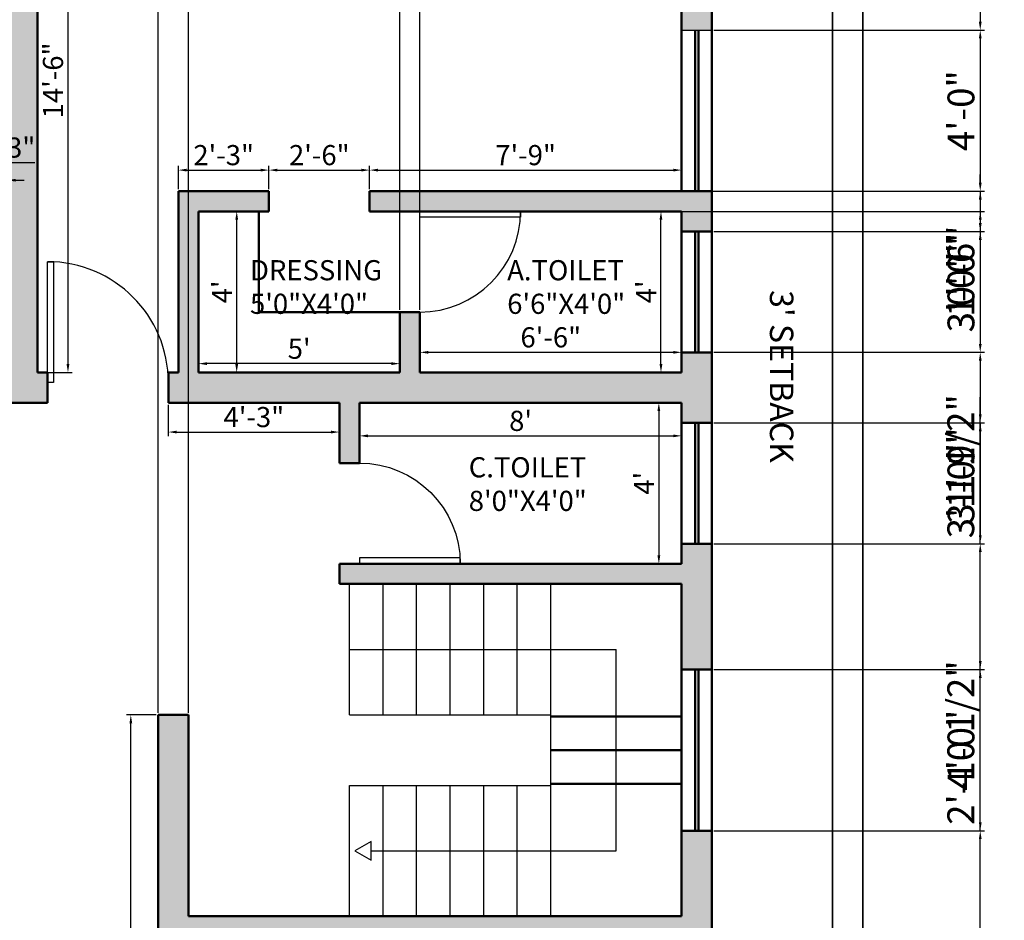
# Model space of a CAD drawing. Units: inches. Extents: x 2442 to 3851, y 589 to 2836.
# Tile 21 of 22: x 3558 to 3851, y 2400 to 2668. Entities that reach past the tile are written whole.
import ezdxf

# ---------------------------------------------------------------- set-up
doc = ezdxf.new("R2010")
doc.units = ezdxf.units.IN
for name, color, linetype, lineweight in [('A-ANNO-DIMS', 2, 'Continuous', 18), ('A-ANNO-TEXT', 7, 'Continuous', 18), ('A-AREA-IDEN', 7, 'Continuous', 18), ('A-DOOR', 4, 'Continuous', 25), ('A-FLOR-STRS', 3, 'Continuous', 25), ('A-GLAZ', 1, 'Continuous', 25), ('A-WALL', 7, 'Continuous', 50), ('A-WALL-PATT', 8, 'Continuous', 13), ('C-PROP', 7, 'Continuous', 35)]:
    doc.layers.add(name, color=color, linetype=linetype, lineweight=lineweight)
doc.styles.get("Standard").update_dxf_attribs({"font": 'arial.ttf'})
doc.dimstyles.new('ISO-25', dxfattribs={"dimtxt": 8, "dimasz": 2.5, "dimexe": 1.25, "dimexo": 0.625, "dimtad": 1, "dimlunit": 3, "dimtxsty": 'Standard', "dimcen": 2.5, "dimadec": 0, "dimazin": 0, "dimtfac": 1, "dimtmove": 0, "dimatfit": 3, "dimfxl": 1, "dimarcsym": 0})

# ---------------------------------------------------------------- blocks, each defined once
blk = doc.blocks.new('*U23')
for p, q in [((0, 0), (0, -6)), ((36, 0), (36, -6))]:
    blk.add_line(p, q)
blk.add_lwpolyline([(0, 0), (0, 36), (1.75, 36), (1.75, 0)], close=True)
blk.add_arc((0, 0), 36, 0, 90)
blk = doc.blocks.new('*U24')
for p, q in [((0, 0), (0, -6)), ((30, 0), (30, -6))]:
    blk.add_line(p, q)
blk.add_lwpolyline([(0, 0), (0, 30), (1.75, 30), (1.75, 0)], close=True)
blk.add_arc((0, 0), 30, 0, 90)
blk = doc.blocks.new('*D104')
at = {"layer": 'A-ANNO-DIMS', "color": 0, "lineweight": -2, "transparency": 16777216}
for p, q in [((3552.52, 2620.49), (3554.1, 2625.74)), ((3554.1, 2625.74), (3562.24, 2625.74)), ((3551.02, 2617.83), (3551.02, 2621.74)), ((3554.02, 2617.83), (3554.02, 2621.74)), ((3548.52, 2620.49), (3546.02, 2620.49)), ((3551.02, 2620.49), (3554.02, 2620.49)), ((3551.02, 2620.49), (3554.02, 2620.49)), ((3556.52, 2620.49), (3559.02, 2620.49))]:
    blk.add_line(p, q, dxfattribs=at)
at = {"layer": 'A-ANNO-DIMS', "color": 0, "transparency": 16777216}
for points in [[(3548.52, 2620.9), (3548.52, 2620.07), (3551.02, 2620.49)], [(3556.52, 2620.9), (3556.52, 2620.07), (3554.02, 2620.49)]]:
    blk.add_solid(points, dxfattribs=at)
at = {"layer": 'Defpoints', "color": 0, "transparency": 16777216}
for p in [(3554.02, 2620.49), (3551.02, 2617.21), (3554.02, 2617.21)]:
    blk.add_point(p, dxfattribs=at)
at = {"layer": 'A-ANNO-DIMS', "color": 0, "transparency": 16777216, "insert": (3558.17, 2629.43), "char_height": 6, "attachment_point": 5}
blk.add_mtext('3"', dxfattribs=at)
blk = doc.blocks.new('*D117')
at = {"layer": 'A-ANNO-DIMS', "color": 0, "lineweight": -2, "transparency": 16777216}
for p, q in [((3563.65, 2737.21), (3573.36, 2737.21)), ((3572.11, 2734.71), (3572.11, 2565.71)), ((3563.65, 2563.21), (3573.36, 2563.21))]:
    blk.add_line(p, q, dxfattribs=at)
at = {"layer": 'A-ANNO-DIMS', "color": 0, "transparency": 16777216}
for points in [[(3571.69, 2734.71), (3572.53, 2734.71), (3572.11, 2737.21)], [(3571.69, 2565.71), (3572.53, 2565.71), (3572.11, 2563.21)]]:
    blk.add_solid(points, dxfattribs=at)
at = {"layer": 'Defpoints', "color": 0, "transparency": 16777216}
for p in [(3563.02, 2737.21), (3563.02, 2563.21), (3572.11, 2563.21)]:
    blk.add_point(p, dxfattribs=at)
at = {"layer": 'A-ANNO-DIMS', "color": 0, "transparency": 16777216, "insert": (3568.42, 2650.21), "char_height": 6, "attachment_point": 5, "rotation": 90}
blk.add_mtext('14\'-6"', dxfattribs=at)
blk = doc.blocks.new('*D118')
at = {"layer": 'A-ANNO-DIMS', "color": 0, "lineweight": -2, "transparency": 16777216}
for p, q in [((3605.02, 2617.83), (3605.02, 2624.74)), ((3632.02, 2617.83), (3632.02, 2624.74)), ((3607.52, 2623.49), (3629.52, 2623.49))]:
    blk.add_line(p, q, dxfattribs=at)
at = {"layer": 'A-ANNO-DIMS', "color": 0, "transparency": 16777216}
for points in [[(3607.52, 2623.91), (3607.52, 2623.07), (3605.02, 2623.49)], [(3629.52, 2623.91), (3629.52, 2623.07), (3632.02, 2623.49)]]:
    blk.add_solid(points, dxfattribs=at)
at = {"layer": 'Defpoints', "color": 0, "transparency": 16777216}
for p in [(3632.02, 2623.49), (3605.02, 2617.21), (3632.02, 2617.21)]:
    blk.add_point(p, dxfattribs=at)
at = {"layer": 'A-ANNO-DIMS', "color": 0, "transparency": 16777216, "insert": (3618.52, 2627.18), "char_height": 6, "attachment_point": 5}
blk.add_mtext('2\'-3"', dxfattribs=at)
blk = doc.blocks.new('*D119')
at = {"layer": 'A-ANNO-DIMS', "color": 0, "lineweight": -2, "transparency": 16777216}
for p, q in [((3632.02, 2617.83), (3632.02, 2624.74)), ((3662.02, 2617.83), (3662.02, 2624.74)), ((3634.52, 2623.49), (3659.52, 2623.49))]:
    blk.add_line(p, q, dxfattribs=at)
at = {"layer": 'A-ANNO-DIMS', "color": 0, "transparency": 16777216}
for points in [[(3634.52, 2623.91), (3634.52, 2623.07), (3632.02, 2623.49)], [(3659.52, 2623.91), (3659.52, 2623.07), (3662.02, 2623.49)]]:
    blk.add_solid(points, dxfattribs=at)
at = {"layer": 'Defpoints', "color": 0, "transparency": 16777216}
for p in [(3662.02, 2623.49), (3632.02, 2617.21), (3662.02, 2617.21)]:
    blk.add_point(p, dxfattribs=at)
at = {"layer": 'A-ANNO-DIMS', "color": 0, "transparency": 16777216, "insert": (3647.02, 2627.18), "char_height": 6, "attachment_point": 5}
blk.add_mtext('2\'-6"', dxfattribs=at)
blk = doc.blocks.new('*D120')
at = {"layer": 'A-ANNO-DIMS', "color": 0, "lineweight": -2, "transparency": 16777216}
for p, q in [((3662.02, 2617.83), (3662.02, 2624.74)), ((3755.02, 2617.83), (3755.02, 2624.74)), ((3664.52, 2623.49), (3752.52, 2623.49))]:
    blk.add_line(p, q, dxfattribs=at)
at = {"layer": 'A-ANNO-DIMS', "color": 0, "transparency": 16777216}
for points in [[(3664.52, 2623.91), (3664.52, 2623.07), (3662.02, 2623.49)], [(3752.52, 2623.91), (3752.52, 2623.07), (3755.02, 2623.49)]]:
    blk.add_solid(points, dxfattribs=at)
at = {"layer": 'Defpoints', "color": 0, "transparency": 16777216}
for p in [(3755.02, 2623.49), (3662.02, 2617.21), (3755.02, 2617.21)]:
    blk.add_point(p, dxfattribs=at)
at = {"layer": 'A-ANNO-DIMS', "color": 0, "transparency": 16777216, "insert": (3708.52, 2627.18), "char_height": 6, "attachment_point": 5}
blk.add_mtext('7\'-9"', dxfattribs=at)
blk = doc.blocks.new('*D121')
at = {"layer": 'A-ANNO-DIMS', "color": 0, "lineweight": -2, "transparency": 16777216}
for p, q in [((3677.02, 2563.83), (3677.02, 2570.46)), ((3679.52, 2569.21), (3752.52, 2569.21)), ((3755.02, 2563.83), (3755.02, 2570.46))]:
    blk.add_line(p, q, dxfattribs=at)
at = {"layer": 'A-ANNO-DIMS', "color": 0, "transparency": 16777216}
for points in [[(3679.52, 2569.62), (3679.52, 2568.79), (3677.02, 2569.21)], [(3752.52, 2569.62), (3752.52, 2568.79), (3755.02, 2569.21)]]:
    blk.add_solid(points, dxfattribs=at)
at = {"layer": 'Defpoints', "color": 0, "transparency": 16777216}
for p in [(3755.02, 2569.21), (3677.02, 2563.21), (3755.02, 2563.21)]:
    blk.add_point(p, dxfattribs=at)
at = {"layer": 'A-ANNO-DIMS', "color": 0, "transparency": 16777216, "insert": (3716.02, 2572.9), "char_height": 6, "attachment_point": 5}
blk.add_mtext('6\'-6"', dxfattribs=at)
blk = doc.blocks.new('*D122')
at = {"layer": 'A-ANNO-DIMS', "color": 0, "lineweight": -2, "transparency": 16777216}
for p, q in [((3754.4, 2611.21), (3747.61, 2611.21)), ((3748.86, 2565.71), (3748.86, 2608.71)), ((3754.4, 2563.21), (3747.61, 2563.21))]:
    blk.add_line(p, q, dxfattribs=at)
at = {"layer": 'A-ANNO-DIMS', "color": 0, "transparency": 16777216}
for points in [[(3748.44, 2608.71), (3749.27, 2608.71), (3748.86, 2611.21)], [(3748.44, 2565.71), (3749.27, 2565.71), (3748.86, 2563.21)]]:
    blk.add_solid(points, dxfattribs=at)
at = {"layer": 'Defpoints', "color": 0, "transparency": 16777216}
for p in [(3748.86, 2611.21), (3755.02, 2611.21), (3755.02, 2563.21)]:
    blk.add_point(p, dxfattribs=at)
at = {"layer": 'A-ANNO-DIMS', "color": 0, "transparency": 16777216, "insert": (3745.23, 2587.21), "char_height": 6, "attachment_point": 5, "rotation": 90}
blk.add_mtext("4'", dxfattribs=at)
blk = doc.blocks.new('*D123')
at = {"layer": 'A-ANNO-DIMS', "color": 0, "lineweight": -2, "transparency": 16777216}
for p, q in [((3611.02, 2563.83), (3611.02, 2567.09)), ((3668.52, 2565.84), (3613.52, 2565.84)), ((3671.02, 2563.83), (3671.02, 2567.09))]:
    blk.add_line(p, q, dxfattribs=at)
at = {"layer": 'A-ANNO-DIMS', "color": 0, "transparency": 16777216}
for points in [[(3613.52, 2566.25), (3613.52, 2565.42), (3611.02, 2565.84)], [(3668.52, 2566.25), (3668.52, 2565.42), (3671.02, 2565.84)]]:
    blk.add_solid(points, dxfattribs=at)
at = {"layer": 'Defpoints', "color": 0, "transparency": 16777216}
for p in [(3611.02, 2565.84), (3611.02, 2563.21), (3671.02, 2563.21)]:
    blk.add_point(p, dxfattribs=at)
at = {"layer": 'A-ANNO-DIMS', "color": 0, "transparency": 16777216, "insert": (3641.02, 2569.51), "char_height": 6, "attachment_point": 5}
blk.add_mtext("5'", dxfattribs=at)
blk = doc.blocks.new('*D124')
at = {"layer": 'A-ANNO-DIMS', "color": 0, "lineweight": -2, "transparency": 16777216}
for p, q in [((3611.65, 2611.21), (3623.65, 2611.21)), ((3622.4, 2565.71), (3622.4, 2608.71)), ((3611.65, 2563.21), (3623.65, 2563.21))]:
    blk.add_line(p, q, dxfattribs=at)
at = {"layer": 'A-ANNO-DIMS', "color": 0, "transparency": 16777216}
for points in [[(3621.99, 2608.71), (3622.82, 2608.71), (3622.4, 2611.21)], [(3621.99, 2565.71), (3622.82, 2565.71), (3622.4, 2563.21)]]:
    blk.add_solid(points, dxfattribs=at)
at = {"layer": 'Defpoints', "color": 0, "transparency": 16777216}
for p in [(3611.02, 2611.21), (3622.4, 2611.21), (3611.02, 2563.21)]:
    blk.add_point(p, dxfattribs=at)
at = {"layer": 'A-ANNO-DIMS', "color": 0, "transparency": 16777216, "insert": (3618.78, 2587.21), "char_height": 6, "attachment_point": 5, "rotation": 90}
blk.add_mtext("4'", dxfattribs=at)
blk = doc.blocks.new('*D125')
at = {"layer": 'A-ANNO-DIMS', "color": 0, "lineweight": -2, "transparency": 16777216}
for p, q in [((3659.02, 2553.58), (3659.02, 2543.08)), ((3755.02, 2553.58), (3755.02, 2543.08)), ((3661.52, 2544.33), (3752.52, 2544.33))]:
    blk.add_line(p, q, dxfattribs=at)
at = {"layer": 'A-ANNO-DIMS', "color": 0, "transparency": 16777216}
for points in [[(3661.52, 2544.74), (3661.52, 2543.91), (3659.02, 2544.33)], [(3752.52, 2544.74), (3752.52, 2543.91), (3755.02, 2544.33)]]:
    blk.add_solid(points, dxfattribs=at)
at = {"layer": 'Defpoints', "color": 0, "transparency": 16777216}
for p in [(3659.02, 2554.21), (3755.02, 2554.21), (3755.02, 2544.33)]:
    blk.add_point(p, dxfattribs=at)
at = {"layer": 'A-ANNO-DIMS', "color": 0, "transparency": 16777216, "insert": (3707.02, 2548.02), "char_height": 6, "attachment_point": 5}
blk.add_mtext("8'", dxfattribs=at)
blk = doc.blocks.new('*D126')
at = {"layer": 'A-ANNO-DIMS', "color": 0, "lineweight": -2, "transparency": 16777216}
for p, q in [((3754.4, 2554.21), (3746.98, 2554.21)), ((3748.23, 2551.71), (3748.23, 2508.71)), ((3754.4, 2506.21), (3746.98, 2506.21))]:
    blk.add_line(p, q, dxfattribs=at)
at = {"layer": 'A-ANNO-DIMS', "color": 0, "transparency": 16777216}
for points in [[(3747.81, 2551.71), (3748.64, 2551.71), (3748.23, 2554.21)], [(3747.81, 2508.71), (3748.64, 2508.71), (3748.23, 2506.21)]]:
    blk.add_solid(points, dxfattribs=at)
at = {"layer": 'Defpoints', "color": 0, "transparency": 16777216}
for p in [(3755.02, 2554.21), (3748.23, 2506.21), (3755.02, 2506.21)]:
    blk.add_point(p, dxfattribs=at)
at = {"layer": 'A-ANNO-DIMS', "color": 0, "transparency": 16777216, "insert": (3744.6, 2530.21), "char_height": 6, "attachment_point": 5, "rotation": 90}
blk.add_mtext("4'", dxfattribs=at)
blk = doc.blocks.new('*D127')
at = {"layer": 'A-ANNO-DIMS', "color": 0, "lineweight": -2, "transparency": 16777216}
for p, q in [((3602.02, 2553.58), (3602.02, 2544.21)), ((3653.02, 2553.58), (3653.02, 2544.21)), ((3604.52, 2545.46), (3650.52, 2545.46))]:
    blk.add_line(p, q, dxfattribs=at)
at = {"layer": 'A-ANNO-DIMS', "color": 0, "transparency": 16777216}
for points in [[(3604.52, 2545.88), (3604.52, 2545.04), (3602.02, 2545.46)], [(3650.52, 2545.88), (3650.52, 2545.04), (3653.02, 2545.46)]]:
    blk.add_solid(points, dxfattribs=at)
at = {"layer": 'Defpoints', "color": 0, "transparency": 16777216}
for p in [(3602.02, 2554.21), (3653.02, 2554.21), (3653.02, 2545.46)]:
    blk.add_point(p, dxfattribs=at)
at = {"layer": 'A-ANNO-DIMS', "color": 0, "transparency": 16777216, "insert": (3627.52, 2549.15), "char_height": 6, "attachment_point": 5}
blk.add_mtext('4\'-3"', dxfattribs=at)
blk = doc.blocks.new('*D133')
at = {"layer": 'A-ANNO-DIMS', "color": 0, "lineweight": -2, "transparency": 16777216}
for p, q in [((3598.4, 2461.21), (3589.59, 2461.21)), ((3590.84, 2259.71), (3590.84, 2458.71)), ((3598.4, 2257.21), (3589.59, 2257.21))]:
    blk.add_line(p, q, dxfattribs=at)
at = {"layer": 'A-ANNO-DIMS', "color": 0, "transparency": 16777216}
for points in [[(3590.43, 2458.71), (3591.26, 2458.71), (3590.84, 2461.21)], [(3590.43, 2259.71), (3591.26, 2259.71), (3590.84, 2257.21)]]:
    blk.add_solid(points, dxfattribs=at)
at = {"layer": 'Defpoints', "color": 0, "transparency": 16777216}
for p in [(3590.84, 2461.21), (3599.02, 2461.21), (3599.02, 2257.21)]:
    blk.add_point(p, dxfattribs=at)
at = {"layer": 'A-ANNO-DIMS', "color": 0, "transparency": 16777216, "insert": (3587.21, 2359.21), "char_height": 6, "attachment_point": 5, "rotation": 90}
blk.add_mtext("17'", dxfattribs=at)
blk = doc.blocks.new('*D227')
at = {"layer": 'A-ANNO-DIMS', "color": 0, "lineweight": -2, "transparency": 16777216}
for p, q in [((3764.65, 2746.21), (3845.27, 2746.21)), ((3844.02, 2743.71), (3844.02, 2667.71)), ((3764.65, 2665.21), (3845.27, 2665.21))]:
    blk.add_line(p, q, dxfattribs=at)
at = {"layer": 'A-ANNO-DIMS', "color": 0, "transparency": 16777216}
for points in [[(3843.61, 2743.71), (3844.44, 2743.71), (3844.02, 2746.21)], [(3843.61, 2667.71), (3844.44, 2667.71), (3844.02, 2665.21)]]:
    blk.add_solid(points, dxfattribs=at)
at = {"layer": 'Defpoints', "color": 0, "transparency": 16777216}
for p in [(3764.02, 2746.21), (3764.02, 2665.21), (3844.02, 2665.21)]:
    blk.add_point(p, dxfattribs=at)
at = {"layer": 'A-ANNO-DIMS', "color": 0, "transparency": 16777216, "insert": (3839.31, 2705.71), "char_height": 8, "attachment_point": 5, "rotation": 90}
blk.add_mtext('6\'-9"', dxfattribs=at)
blk = doc.blocks.new('*D228')
at = {"layer": 'A-ANNO-DIMS', "color": 0, "lineweight": -2, "transparency": 16777216}
for p, q in [((3764.65, 2665.21), (3845.27, 2665.21)), ((3844.02, 2662.71), (3844.02, 2619.71)), ((3764.65, 2617.21), (3845.27, 2617.21))]:
    blk.add_line(p, q, dxfattribs=at)
at = {"layer": 'A-ANNO-DIMS', "color": 0, "transparency": 16777216}
for points in [[(3843.61, 2662.71), (3844.44, 2662.71), (3844.02, 2665.21)], [(3843.61, 2619.71), (3844.44, 2619.71), (3844.02, 2617.21)]]:
    blk.add_solid(points, dxfattribs=at)
at = {"layer": 'Defpoints', "color": 0, "transparency": 16777216}
for p in [(3764.02, 2665.21), (3764.02, 2617.21), (3844.02, 2617.21)]:
    blk.add_point(p, dxfattribs=at)
at = {"layer": 'A-ANNO-DIMS', "color": 0, "transparency": 16777216, "insert": (3839.31, 2641.21), "char_height": 8, "attachment_point": 5, "rotation": 90}
blk.add_mtext('4\'-0"', dxfattribs=at)
blk = doc.blocks.new('*D229')
at = {"layer": 'A-ANNO-DIMS', "color": 0, "lineweight": -2, "transparency": 16777216}
for p, q in [((3844.02, 2426.71), (3844.02, 2476.72)), ((3764.65, 2426.71), (3845.27, 2426.71)), ((3844.02, 2394.71), (3844.02, 2424.21)), ((3764.65, 2392.21), (3845.27, 2392.21))]:
    blk.add_line(p, q, dxfattribs=at)
at = {"layer": 'A-ANNO-DIMS', "color": 0, "transparency": 16777216}
for points in [[(3843.61, 2424.21), (3844.44, 2424.21), (3844.02, 2426.71)], [(3843.61, 2394.71), (3844.44, 2394.71), (3844.02, 2392.21)]]:
    blk.add_solid(points, dxfattribs=at)
at = {"layer": 'Defpoints', "color": 0, "transparency": 16777216}
for p in [(3764.02, 2426.71), (3844.02, 2426.71), (3764.02, 2392.21)]:
    blk.add_point(p, dxfattribs=at)
at = {"layer": 'A-ANNO-DIMS', "color": 0, "transparency": 16777216, "insert": (3839.26, 2452.96), "char_height": 8, "attachment_point": 5, "rotation": 90}
blk.add_mtext('2\'-10 1/2"', dxfattribs=at)
blk = doc.blocks.new('*D230')
at = {"layer": 'A-ANNO-DIMS', "color": 0, "lineweight": -2, "transparency": 16777216}
for p, q in [((3764.65, 2474.71), (3845.27, 2474.71)), ((3844.02, 2429.21), (3844.02, 2472.21)), ((3764.65, 2426.71), (3845.27, 2426.71))]:
    blk.add_line(p, q, dxfattribs=at)
at = {"layer": 'A-ANNO-DIMS', "color": 0, "transparency": 16777216}
for points in [[(3843.61, 2472.21), (3844.44, 2472.21), (3844.02, 2474.71)], [(3843.61, 2429.21), (3844.44, 2429.21), (3844.02, 2426.71)]]:
    blk.add_solid(points, dxfattribs=at)
at = {"layer": 'Defpoints', "color": 0, "transparency": 16777216}
for p in [(3764.02, 2474.71), (3844.02, 2474.71), (3764.02, 2426.71)]:
    blk.add_point(p, dxfattribs=at)
at = {"layer": 'A-ANNO-DIMS', "color": 0, "transparency": 16777216, "insert": (3839.31, 2450.71), "char_height": 8, "attachment_point": 5, "rotation": 90}
blk.add_mtext('4\'-0"', dxfattribs=at)
blk = doc.blocks.new('*D231')
at = {"layer": 'A-ANNO-DIMS', "color": 0, "lineweight": -2, "transparency": 16777216}
for p, q in [((3844.02, 2512.21), (3844.02, 2555.86)), ((3764.65, 2512.21), (3845.27, 2512.21)), ((3844.02, 2477.21), (3844.02, 2509.71)), ((3764.65, 2474.71), (3845.27, 2474.71))]:
    blk.add_line(p, q, dxfattribs=at)
at = {"layer": 'A-ANNO-DIMS', "color": 0, "transparency": 16777216}
for points in [[(3843.61, 2509.71), (3844.44, 2509.71), (3844.02, 2512.21)], [(3843.61, 2477.21), (3844.44, 2477.21), (3844.02, 2474.71)]]:
    blk.add_solid(points, dxfattribs=at)
at = {"layer": 'Defpoints', "color": 0, "transparency": 16777216}
for p in [(3764.02, 2512.21), (3844.02, 2512.21), (3764.02, 2474.71)]:
    blk.add_point(p, dxfattribs=at)
at = {"layer": 'A-ANNO-DIMS', "color": 0, "transparency": 16777216, "insert": (3839.26, 2535.28), "char_height": 8, "attachment_point": 5, "rotation": 90}
blk.add_mtext('3\'-1 1/2"', dxfattribs=at)
blk = doc.blocks.new('*D232')
at = {"layer": 'A-ANNO-DIMS', "color": 0, "lineweight": -2, "transparency": 16777216}
for p, q in [((3764.65, 2617.21), (3845.27, 2617.21)), ((3844.02, 2614.71), (3844.02, 2607.71)), ((3764.65, 2605.21), (3845.27, 2605.21)), ((3844.02, 2605.21), (3844.02, 2580.94))]:
    blk.add_line(p, q, dxfattribs=at)
at = {"layer": 'A-ANNO-DIMS', "color": 0, "transparency": 16777216}
for points in [[(3843.61, 2614.71), (3844.44, 2614.71), (3844.02, 2617.21)], [(3843.61, 2607.71), (3844.44, 2607.71), (3844.02, 2605.21)]]:
    blk.add_solid(points, dxfattribs=at)
at = {"layer": 'Defpoints', "color": 0, "transparency": 16777216}
for p in [(3764.02, 2617.21), (3764.02, 2605.21), (3844.02, 2605.21)]:
    blk.add_point(p, dxfattribs=at)
at = {"layer": 'A-ANNO-DIMS', "color": 0, "transparency": 16777216, "insert": (3839.31, 2591.83), "char_height": 8, "attachment_point": 5, "rotation": 90}
blk.add_mtext('1\'-0"', dxfattribs=at)
blk = doc.blocks.new('*D233')
at = {"layer": 'A-ANNO-DIMS', "color": 0, "lineweight": -2, "transparency": 16777216}
for p, q in [((3764.65, 2605.21), (3845.27, 2605.21)), ((3844.02, 2602.71), (3844.02, 2571.71)), ((3764.65, 2569.21), (3845.27, 2569.21))]:
    blk.add_line(p, q, dxfattribs=at)
at = {"layer": 'A-ANNO-DIMS', "color": 0, "transparency": 16777216}
for points in [[(3843.61, 2602.71), (3844.44, 2602.71), (3844.02, 2605.21)], [(3843.61, 2571.71), (3844.44, 2571.71), (3844.02, 2569.21)]]:
    blk.add_solid(points, dxfattribs=at)
at = {"layer": 'Defpoints', "color": 0, "transparency": 16777216}
for p in [(3764.02, 2605.21), (3764.02, 2569.21), (3844.02, 2569.21)]:
    blk.add_point(p, dxfattribs=at)
at = {"layer": 'A-ANNO-DIMS', "color": 0, "transparency": 16777216, "insert": (3839.31, 2587.21), "char_height": 8, "attachment_point": 5, "rotation": 90}
blk.add_mtext('3\'-0"', dxfattribs=at)
blk = doc.blocks.new('*D234')
at = {"layer": 'A-ANNO-DIMS', "color": 0, "lineweight": -2, "transparency": 16777216}
for p, q in [((3764.65, 2569.21), (3845.27, 2569.21)), ((3844.02, 2566.71), (3844.02, 2550.71)), ((3764.65, 2548.21), (3845.27, 2548.21)), ((3844.02, 2548.21), (3844.02, 2523.94))]:
    blk.add_line(p, q, dxfattribs=at)
at = {"layer": 'A-ANNO-DIMS', "color": 0, "transparency": 16777216}
for points in [[(3843.61, 2566.71), (3844.44, 2566.71), (3844.02, 2569.21)], [(3843.61, 2550.71), (3844.44, 2550.71), (3844.02, 2548.21)]]:
    blk.add_solid(points, dxfattribs=at)
at = {"layer": 'Defpoints', "color": 0, "transparency": 16777216}
for p in [(3764.02, 2569.21), (3764.02, 2548.21), (3844.02, 2548.21)]:
    blk.add_point(p, dxfattribs=at)
at = {"layer": 'A-ANNO-DIMS', "color": 0, "transparency": 16777216, "insert": (3839.31, 2534.83), "char_height": 8, "attachment_point": 5, "rotation": 90}
blk.add_mtext('1\'-9"', dxfattribs=at)
blk = doc.blocks.new('*D235')
at = {"layer": 'A-ANNO-DIMS', "color": 0, "lineweight": -2, "transparency": 16777216}
for p, q in [((3764.65, 2548.21), (3845.27, 2548.21)), ((3844.02, 2545.71), (3844.02, 2514.71)), ((3764.65, 2512.21), (3845.27, 2512.21))]:
    blk.add_line(p, q, dxfattribs=at)
at = {"layer": 'A-ANNO-DIMS', "color": 0, "transparency": 16777216}
for points in [[(3843.61, 2545.71), (3844.44, 2545.71), (3844.02, 2548.21)], [(3843.61, 2514.71), (3844.44, 2514.71), (3844.02, 2512.21)]]:
    blk.add_solid(points, dxfattribs=at)
at = {"layer": 'Defpoints', "color": 0, "transparency": 16777216}
for p in [(3764.02, 2548.21), (3764.02, 2512.21), (3844.02, 2512.21)]:
    blk.add_point(p, dxfattribs=at)
at = {"layer": 'A-ANNO-DIMS', "color": 0, "transparency": 16777216, "insert": (3839.31, 2530.21), "char_height": 8, "attachment_point": 5, "rotation": 90}
blk.add_mtext('3\'-0"', dxfattribs=at)
blk = doc.blocks.new('*D253')
at = {"layer": 'A-ANNO-DIMS', "color": 0, "lineweight": -2, "transparency": 16777216}
for p, q in [((3599.02, 2461.83), (3599.02, 2827.46)), ((3601.52, 2826.21), (3605.52, 2826.21)), ((3608.02, 2461.83), (3608.02, 2827.46)), ((3608.02, 2826.21), (3633.04, 2826.21))]:
    blk.add_line(p, q, dxfattribs=at)
at = {"layer": 'A-ANNO-DIMS', "color": 0, "transparency": 16777216}
for points in [[(3601.52, 2826.62), (3601.52, 2825.79), (3599.02, 2826.21)], [(3605.52, 2826.62), (3605.52, 2825.79), (3608.02, 2826.21)]]:
    blk.add_solid(points, dxfattribs=at)
at = {"layer": 'Defpoints', "color": 0, "transparency": 16777216}
for p in [(3608.02, 2826.21), (3599.02, 2461.21), (3608.02, 2461.21)]:
    blk.add_point(p, dxfattribs=at)
at = {"layer": 'A-ANNO-DIMS', "color": 0, "transparency": 16777216, "insert": (3621.78, 2830.92), "char_height": 8, "attachment_point": 5}
blk.add_mtext('0\'-9"', dxfattribs=at)
blk = doc.blocks.new('*D254')
at = {"layer": 'A-ANNO-DIMS', "color": 0, "lineweight": -2, "transparency": 16777216}
for p, q in [((3668.52, 2826.21), (3666.02, 2826.21)), ((3671.02, 2581.83), (3671.02, 2827.46)), ((3671.02, 2826.21), (3677.02, 2826.21)), ((3677.02, 2581.83), (3677.02, 2827.46)), ((3679.52, 2826.21), (3704.54, 2826.21))]:
    blk.add_line(p, q, dxfattribs=at)
at = {"layer": 'A-ANNO-DIMS', "color": 0, "transparency": 16777216}
for points in [[(3668.52, 2826.62), (3668.52, 2825.79), (3671.02, 2826.21)], [(3679.52, 2826.62), (3679.52, 2825.79), (3677.02, 2826.21)]]:
    blk.add_solid(points, dxfattribs=at)
at = {"layer": 'Defpoints', "color": 0, "transparency": 16777216}
for p in [(3677.02, 2826.21), (3671.02, 2581.21), (3677.02, 2581.21)]:
    blk.add_point(p, dxfattribs=at)
at = {"layer": 'A-ANNO-DIMS', "color": 0, "transparency": 16777216, "insert": (3693.28, 2830.92), "char_height": 8, "attachment_point": 5}
blk.add_mtext('0\'-6"', dxfattribs=at)
blk = doc.blocks.new('*D255')
at = {"layer": 'A-ANNO-DIMS', "color": 0, "lineweight": -2, "transparency": 16777216}
for p, q in [((3844.02, 2619.71), (3844.02, 2622.21)), ((3662.65, 2617.21), (3845.27, 2617.21)), ((3844.02, 2617.21), (3844.02, 2611.21)), ((3662.65, 2611.21), (3845.27, 2611.21)), ((3844.02, 2608.71), (3844.02, 2583.69))]:
    blk.add_line(p, q, dxfattribs=at)
at = {"layer": 'A-ANNO-DIMS', "color": 0, "transparency": 16777216}
for points in [[(3843.61, 2619.71), (3844.44, 2619.71), (3844.02, 2617.21)], [(3843.61, 2608.71), (3844.44, 2608.71), (3844.02, 2611.21)]]:
    blk.add_solid(points, dxfattribs=at)
at = {"layer": 'Defpoints', "color": 0, "transparency": 16777216}
for p in [(3662.02, 2617.21), (3662.02, 2611.21), (3844.02, 2611.21)]:
    blk.add_point(p, dxfattribs=at)
at = {"layer": 'A-ANNO-DIMS', "color": 0, "transparency": 16777216, "insert": (3839.31, 2594.95), "char_height": 8, "attachment_point": 5, "rotation": 90}
blk.add_mtext('0\'-6"', dxfattribs=at)

msp = doc.modelspace()

# ---------------------------------------------------------------- hatches: boundary and pattern name
at = {"layer": 'A-WALL-PATT'}
h = msp.add_hatch(color=256, dxfattribs=at)
h.dxf.hatch_style = 1
h.paths.add_polyline_path([(3356.024, 2713.208), (3356.024, 2719.208), (3356.024, 2722.208), (3254.024, 2722.208), (3254.024, 2657.708), (3263.024, 2657.708), (3263.024, 2713.208)])
h.paths.add_polyline_path([(3416.024, 2737.208), (3446.024, 2737.208), (3446.024, 2746.208), (3416.024, 2746.208), (3416.024, 2782.208), (3407.024, 2782.208), (3407.024, 2722.208), (3386.024, 2722.208), (3386.024, 2719.208), (3386.024, 2713.208), (3407.024, 2713.208), (3407.024, 2593.208), (3416.024, 2593.208), (3416.024, 2608.208), (3515.024, 2608.208), (3515.024, 2614.208), (3515.024, 2617.208), (3416.024, 2617.208)])
h.paths.add_polyline_path([(3563.024, 2737.208), (3566.024, 2737.208), (3566.024, 2746.208), (3512.024, 2746.208), (3512.024, 2737.208), (3554.024, 2737.208), (3554.024, 2617.208), (3551.024, 2617.208), (3551.024, 2614.208), (3551.024, 2608.208), (3554.024, 2608.208), (3554.024, 2554.208), (3566.024, 2554.208), (3566.024, 2560.208), (3566.024, 2563.208), (3563.024, 2563.208)])
h.paths.add_polyline_path([(3614.024, 2746.208), (3614.024, 2737.208), (3683.024, 2737.208), (3683.024, 2746.208)])
h.paths.add_polyline_path([(3755.024, 2737.208), (3755.024, 2665.208), (3764.024, 2665.208), (3764.024, 2746.208), (3731.024, 2746.208), (3731.024, 2737.208)])
h.paths.add_polyline_path([(3662.024, 2617.208), (3662.024, 2611.208), (3755.024, 2611.208), (3755.024, 2605.208), (3764.024, 2605.208), (3764.024, 2617.208)])
h.paths.add_polyline_path([(3755.024, 2554.208), (3755.024, 2548.208), (3764.024, 2548.208), (3764.024, 2569.208), (3755.024, 2569.208), (3755.024, 2563.208), (3677.024, 2563.208), (3677.024, 2581.208), (3671.024, 2581.208), (3671.024, 2563.208), (3611.024, 2563.208), (3611.024, 2611.208), (3632.024, 2611.208), (3632.024, 2617.208), (3605.024, 2617.208), (3605.024, 2563.208), (3602.024, 2563.208), (3602.024, 2554.208), (3653.024, 2554.208), (3653.024, 2536.208), (3659.024, 2536.208), (3659.024, 2554.208)])
h.paths.add_polyline_path([(3764.024, 2512.208), (3755.024, 2512.208), (3755.024, 2506.208), (3653.024, 2506.208), (3653.024, 2500.208), (3755.024, 2500.208), (3755.024, 2474.708), (3764.024, 2474.708)])
h.paths.add_polyline_path([(3608.024, 2392.208), (3764.024, 2392.208), (3764.024, 2426.708), (3755.024, 2426.708), (3755.024, 2401.208), (3608.024, 2401.208), (3608.024, 2461.208), (3599.024, 2461.208), (3599.024, 2353.208), (3608.024, 2353.208)])
h.paths.add_polyline_path([(3410.024, 2401.208), (3263.024, 2401.208), (3263.024, 2473.208), (3254.024, 2473.208), (3254.024, 2368.208), (3263.024, 2368.208), (3263.024, 2392.208), (3410.024, 2392.208), (3410.024, 2344.208), (3419.024, 2344.208), (3419.024, 2506.208), (3413.024, 2506.208), (3410.024, 2506.208)])
h.paths.add_polyline_path([(3263.024, 2609.708), (3254.024, 2609.708), (3254.024, 2521.208), (3263.024, 2521.208), (3263.024, 2545.208), (3410.024, 2545.208), (3410.024, 2542.208), (3413.024, 2542.208), (3419.024, 2542.208), (3419.024, 2557.208), (3407.024, 2557.208), (3407.024, 2554.208), (3263.024, 2554.208)])
h.paths.add_polyline_path([(3254.024, 2191.208), (3263.024, 2191.208), (3263.024, 2287.208), (3269.024, 2287.208), (3269.024, 2293.208), (3269.024, 2296.208), (3263.024, 2296.208), (3263.024, 2320.208), (3254.024, 2320.208)])
h.paths.add_polyline_path([(3419.024, 2296.208), (3386.024, 2296.208), (3386.024, 2287.208), (3410.024, 2287.208), (3410.024, 2191.208), (3419.024, 2191.208), (3419.024, 2248.208), (3449.024, 2248.208), (3449.024, 2257.208), (3419.024, 2257.208)])
h.paths.add_polyline_path([(3581.024, 2248.208), (3608.024, 2248.208), (3608.024, 2287.208), (3599.024, 2287.208), (3599.024, 2257.208), (3581.024, 2257.208)])
h.paths.add_polyline_path([(3491.024, 2248.208), (3515.024, 2248.208), (3515.024, 2257.208), (3491.024, 2257.208)])
h.paths.add_polyline_path([(3320.024, 2296.208), (3309.024, 2296.208), (3309.024, 2287.208), (3320.024, 2287.208)])
h.paths.add_polyline_path([(3282.007, 2631.263), (3387.059, 2631.263), (3387.059, 2661.678), (3282.007, 2661.678)], flags=9)
h.paths.add_polyline_path([(3511.253, 2214.916), (3571.545, 2214.916), (3571.545, 2229.862), (3511.253, 2229.862)], flags=9)
h.paths.add_polyline_path([(3777.335, 2589.915), (3777.335, 2529.623), (3792.281, 2529.623), (3792.281, 2589.915)], flags=9)
h.paths.add_polyline_path([(3558.97, 2754.629), (3619.262, 2754.629), (3619.262, 2769.575), (3558.97, 2769.575)], flags=9)
h.paths.add_polyline_path([(3314.979, 2749.318), (3377.263, 2749.318), (3377.263, 2779.733), (3314.979, 2779.733)], flags=9)
h.paths.add_polyline_path([(3624.453, 2577.252), (3671.045, 2577.252), (3671.045, 2600.063), (3624.453, 2600.063)], flags=25)
h.paths.add_polyline_path([(3701.15, 2577.252), (3744.07, 2577.252), (3744.07, 2600.063), (3701.15, 2600.063)], flags=25)
h.paths.add_polyline_path([(3689.533, 2518.545), (3731.868, 2518.545), (3731.868, 2541.356), (3689.533, 2541.356)], flags=9)
h.paths.add_polyline_path([(3629.196, 2666.979), (3693.452, 2666.979), (3693.452, 2697.394), (3629.196, 2697.394)], flags=9)
h.paths.add_polyline_path([(3441.284, 2669.891), (3505.54, 2669.891), (3505.54, 2700.306), (3441.284, 2700.306)], flags=25)
h.paths.add_polyline_path([(3306.565, 2459.233), (3370.821, 2459.233), (3370.821, 2489.648), (3306.565, 2489.648)], flags=25)
h.paths.add_polyline_path([(3307.889, 2320.733), (3387.355, 2320.733), (3387.355, 2351.148), (3307.889, 2351.148)], flags=9)
h.paths.add_polyline_path([(3452.987, 2372.794), (3554.971, 2372.794), (3554.971, 2403.208), (3452.987, 2403.208)], flags=9)

# ---------------------------------------------------------------- linework, layer by layer
at = {"layer": 'A-FLOR-STRS'}
for p, q in [((3656.024, 2461.208), (3656.024, 2500.208)), ((3666.024, 2461.208), (3666.024, 2500.208)), ((3676.024, 2461.208), (3676.024, 2500.208)), ((3686.024, 2461.208), (3686.024, 2500.208)), ((3696.024, 2461.208), (3696.024, 2500.208)), ((3706.024, 2461.208), (3706.024, 2500.208)), ((3716.024, 2440.208), (3716.024, 2500.208)), ((3656.024, 2480.708), (3735.524, 2480.708)), ((3735.524, 2420.708), (3735.524, 2480.708)), ((3656.024, 2461.208), (3716.024, 2461.208)), ((3656.024, 2440.208), (3716.024, 2440.208)), ((3662.482, 2420.708), (3735.524, 2420.708))]:
    msp.add_line(p, q, dxfattribs=at)
at = {"layer": 'A-FLOR-STRS', "ltscale": 0.5}
for p, q in [((3656.024, 2401.208), (3656.024, 2440.208)), ((3666.024, 2401.208), (3666.024, 2440.208)), ((3676.024, 2401.208), (3676.024, 2440.208)), ((3686.024, 2401.208), (3686.024, 2440.208)), ((3696.024, 2401.208), (3696.024, 2440.208)), ((3706.024, 2401.208), (3706.024, 2440.208)), ((3716.024, 2401.208), (3716.024, 2440.208))]:
    msp.add_line(p, q, dxfattribs=at)
at = {"layer": 'A-FLOR-STRS'}
msp.add_lwpolyline([(3657.639, 2420.708), (3662.482, 2417.911), (3662.482, 2423.504)], close=True, dxfattribs=at)
at = {"layer": 'A-GLAZ'}
msp.add_line((3755.024, 2665.208), (3764.024, 2665.208), dxfattribs=at)
at = {"layer": 'A-WALL'}
for p, q in [((3764.024, 2392.208), (3764.024, 2746.208)), ((3563.024, 2563.208), (3563.024, 2737.208)), ((3755.024, 2617.208), (3755.024, 2737.208)), ((3759.024, 2617.208), (3759.024, 2665.208)), ((3760.024, 2617.208), (3760.024, 2665.208)), ((3605.024, 2563.208), (3605.024, 2617.208)), ((3605.024, 2617.208), (3632.024, 2617.208)), ((3632.024, 2611.208), (3632.024, 2617.208)), ((3662.024, 2611.208), (3662.024, 2617.208)), ((3662.024, 2617.208), (3764.024, 2617.208)), ((3611.024, 2563.208), (3611.024, 2611.208)), ((3611.024, 2611.208), (3632.024, 2611.208)), ((3629.024, 2581.208), (3629.024, 2611.208)), ((3662.024, 2611.208), (3755.024, 2611.208)), ((3755.024, 2563.208), (3755.024, 2611.208)), ((3755.024, 2605.208), (3764.024, 2605.208)), ((3759.024, 2569.208), (3759.024, 2605.208)), ((3760.024, 2569.208), (3760.024, 2605.208)), ((3629.024, 2581.208), (3671.024, 2581.208)), ((3671.024, 2563.208), (3671.024, 2581.208)), ((3671.024, 2581.208), (3677.024, 2581.208)), ((3677.024, 2563.208), (3677.024, 2581.208)), ((3755.024, 2569.208), (3764.024, 2569.208)), ((3563.024, 2563.208), (3566.024, 2563.208)), ((3566.024, 2554.208), (3566.024, 2563.208)), ((3602.024, 2554.208), (3602.024, 2563.208)), ((3602.024, 2563.208), (3605.024, 2563.208)), ((3611.024, 2563.208), (3671.024, 2563.208)), ((3677.024, 2563.208), (3755.024, 2563.208)), ((3554.024, 2554.208), (3566.024, 2554.208)), ((3602.024, 2554.208), (3653.024, 2554.208)), ((3653.024, 2536.208), (3653.024, 2554.208)), ((3659.024, 2536.208), (3659.024, 2554.208)), ((3659.024, 2554.208), (3755.024, 2554.208)), ((3755.024, 2506.208), (3755.024, 2554.208)), ((3755.024, 2548.208), (3764.024, 2548.208)), ((3759.024, 2512.208), (3759.024, 2548.208)), ((3760.024, 2512.208), (3760.024, 2548.208)), ((3653.024, 2536.208), (3659.024, 2536.208)), ((3755.024, 2512.208), (3764.024, 2512.208)), ((3653.024, 2500.208), (3653.024, 2506.208)), ((3653.024, 2506.208), (3755.024, 2506.208)), ((3653.024, 2500.208), (3755.024, 2500.208)), ((3755.024, 2401.208), (3755.024, 2500.208)), ((3755.024, 2474.708), (3764.024, 2474.708)), ((3759.024, 2426.708), (3759.024, 2474.708)), ((3760.024, 2426.708), (3760.024, 2474.708)), ((3599.024, 2461.208), (3608.024, 2461.208)), ((3599.024, 2257.208), (3599.024, 2461.208)), ((3608.024, 2401.208), (3608.024, 2461.208)), ((3716.024, 2460.708), (3755.024, 2460.708)), ((3716.024, 2450.708), (3755.024, 2450.708)), ((3716.024, 2440.708), (3755.024, 2440.708)), ((3755.024, 2426.708), (3764.024, 2426.708)), ((3608.024, 2401.208), (3755.024, 2401.208))]:
    msp.add_line(p, q, dxfattribs=at)
at = {"layer": 'C-PROP'}
for points in [[(3809.024, 2191.208), (3809.024, 2791.208), (3209.024, 2791.208), (3209.024, 2191.208), (3809.024, 2191.208)], [(3800.024, 2200.208), (3800.024, 2782.208), (3218.024, 2782.208), (3218.024, 2200.208), (3254.024, 2200.208)]]:
    msp.add_lwpolyline(points, dxfattribs=at)

# ---------------------------------------------------------------- block references
at = {"layer": 'A-DOOR', "rotation": 269.9999999999969}
msp.add_blockref('*U24', (3677.024, 2611.208), dxfattribs=at)
at = {"layer": 'A-DOOR'}
msp.add_blockref('*U23', (3566.024, 2560.208), dxfattribs=at)
at = {"layer": 'A-DOOR', "xscale": -1, "rotation": 270}
msp.add_blockref('*U24', (3659.024, 2506.208), dxfattribs=at)

# ---------------------------------------------------------------- texts
at = {"layer": 'A-ANNO-TEXT', "insert": (3788.321, 2587.746), "char_height": 7, "attachment_point": 1, "rotation": 270}
msp.add_mtext_dynamic_manual_height_columns("{\\fTimes New Roman|b0|i0|c0|p18;3' SETBACK}", width=79.56037, gutter_width=12.5, heights=[0], dxfattribs=at)
at = {"layer": 'A-AREA-IDEN', "char_height": 6, "attachment_point": 1}
for s, insert in [('{\\fTimes New Roman|b0|i0|c0|p18;DRESSING\\P5\'0"X4\'0"}', (3626.377, 2596.668)), ('{\\fTimes New Roman|b0|i0|c0|p18;A.TOILET\\P6\'6"X4\'0"}', (3703.031, 2596.668)), ('{\\fTimes New Roman|b0|i0|c0|p18;C.TOILET\\P8\'0"X4\'0"}', (3691.569, 2537.962))]:
    msp.add_mtext_dynamic_manual_height_columns(s, width=110.76054, gutter_width=12.5, heights=[0], dxfattribs=dict(at, insert=insert))

# ---------------------------------------------------------------- dimensions: what is measured, and where the dimension line sits
at = {"layer": 'A-ANNO-DIMS'}
for base, p1, p2, override, picture, middle in [((3608.024, 2826.208), (3599.024, 2461.208), (3608.024, 2461.208), {"dimdec": 1, "dimlfac": 1, "dimrnd": 0, "dimzin": 1, "dimdsep": 46, "dimlunit": 4, "dimfrac": 2}, '*D253', (3621.783, 2830.917)), ((3677.024, 2826.208), (3671.024, 2581.208), (3677.024, 2581.208), {"dimdec": 1, "dimlfac": 1, "dimrnd": 0, "dimzin": 1, "dimdsep": 46, "dimlunit": 4, "dimfrac": 2}, '*D254', (3693.283, 2830.917)), ((3554.024, 2620.486), (3551.024, 2617.208), (3554.024, 2617.208), {"dimtxt": 6, "dimclrd": 0, "dimclre": 0, "dimclrt": 0, "dimtmove": 1}, '*D104', (3554.725, 2629.429)), ((3632.024, 2623.489), (3605.024, 2617.208), (3632.024, 2617.208), {"dimtxt": 6, "dimclrd": 0, "dimclre": 0, "dimclrt": 0}, '*D118', (3618.524, 2627.18)), ((3662.024, 2623.489), (3632.024, 2617.208), (3662.024, 2617.208), {"dimtxt": 6, "dimclrd": 0, "dimclre": 0, "dimclrt": 0, "dimtmove": 1}, '*D119', (3647.024, 2627.178)), ((3755.024, 2623.489), (3662.024, 2617.208), (3755.024, 2617.208), {"dimtxt": 6, "dimclrd": 0, "dimclre": 0, "dimclrt": 0, "dimtmove": 1}, '*D120', (3708.524, 2627.178)), ((3755.024, 2569.208), (3677.024, 2563.208), (3755.024, 2563.208), {"dimtxt": 6, "dimclrd": 0, "dimclre": 0, "dimclrt": 0}, '*D121', (3716.024, 2572.896)), ((3611.024, 2565.836), (3671.024, 2563.208), (3611.024, 2563.208), {"dimtxt": 6, "dimclrd": 0, "dimclre": 0, "dimclrt": 0}, '*D123', (3641.024, 2569.512)), ((3653.024, 2545.461), (3602.024, 2554.208), (3653.024, 2554.208), {"dimtxt": 6, "dimclrd": 0, "dimclre": 0, "dimclrt": 0}, '*D127', (3627.524, 2549.151)), ((3755.024, 2544.327), (3659.024, 2554.208), (3755.024, 2554.208), {"dimtxt": 6, "dimclrd": 0, "dimclre": 0, "dimclrt": 0}, '*D125', (3707.024, 2548.015))]:
    dim = msp.add_linear_dim(base=base, p1=p1, p2=p2, dimstyle='ISO-25', override=override, dxfattribs=at)
    dim.commit()
    dim.dimension.update_dxf_attribs({"geometry": picture, "text_midpoint": middle})
for base, p1, p2, override, picture, middle in [((3844.024, 2665.208), (3764.024, 2746.208), (3764.024, 2665.208), {"dimdec": 1, "dimlfac": 1, "dimrnd": 0, "dimzin": 1, "dimdsep": 46, "dimlunit": 4, "dimfrac": 2}, '*D227', (3839.315, 2705.708)), ((3572.11, 2563.208), (3563.024, 2737.208), (3563.024, 2563.208), {"dimtxt": 6, "dimclrd": 0, "dimclre": 0, "dimclrt": 0}, '*D117', (3568.422, 2650.208)), ((3844.024, 2617.208), (3764.024, 2665.208), (3764.024, 2617.208), {"dimdec": 1, "dimlfac": 1, "dimrnd": 0, "dimzin": 1, "dimdsep": 46, "dimlunit": 4, "dimfrac": 2}, '*D228', (3839.315, 2641.208)), ((3844.024, 2611.208), (3662.024, 2617.208), (3662.024, 2611.208), {"dimdec": 1, "dimlfac": 1, "dimrnd": 0, "dimzin": 1, "dimdsep": 46, "dimlunit": 4, "dimfrac": 2}, '*D255', (3839.315, 2594.95)), ((3844.024, 2605.208), (3764.024, 2617.208), (3764.024, 2605.208), {"dimdec": 1, "dimlfac": 1, "dimrnd": 0, "dimzin": 1, "dimdsep": 46, "dimlunit": 4, "dimfrac": 2}, '*D232', (3839.315, 2591.826)), ((3622.405, 2611.208), (3611.024, 2563.208), (3611.024, 2611.208), {"dimtxt": 6, "dimclrd": 0, "dimclre": 0, "dimclrt": 0}, '*D124', (3618.78, 2587.208)), ((3748.858, 2611.208), (3755.024, 2563.208), (3755.024, 2611.208), {"dimtxt": 6, "dimclrd": 0, "dimclre": 0, "dimclrt": 0}, '*D122', (3745.233, 2587.208)), ((3844.024, 2569.208), (3764.024, 2605.208), (3764.024, 2569.208), {"dimdec": 1, "dimlfac": 1, "dimrnd": 0, "dimzin": 1, "dimdsep": 46, "dimlunit": 4, "dimfrac": 2}, '*D233', (3839.312, 2587.208)), ((3844.024, 2548.208), (3764.024, 2569.208), (3764.024, 2548.208), {"dimdec": 1, "dimlfac": 1, "dimrnd": 0, "dimzin": 1, "dimdsep": 46, "dimlunit": 4, "dimfrac": 2}, '*D234', (3839.315, 2534.826)), ((3748.227, 2506.208), (3755.024, 2554.208), (3755.024, 2506.208), {"dimtxt": 6, "dimclrd": 0, "dimclre": 0, "dimclrt": 0}, '*D126', (3744.602, 2530.208)), ((3844.024, 2512.208), (3764.024, 2474.708), (3764.024, 2512.208), {"dimdec": 1, "dimlfac": 1, "dimrnd": 0, "dimzin": 1, "dimdsep": 46, "dimlunit": 4, "dimfrac": 2}, '*D231', (3839.26, 2535.283)), ((3844.024, 2512.208), (3764.024, 2548.208), (3764.024, 2512.208), {"dimdec": 1, "dimlfac": 1, "dimrnd": 0, "dimzin": 1, "dimdsep": 46, "dimlunit": 4, "dimfrac": 2}, '*D235', (3839.312, 2530.208)), ((3844.024, 2426.708), (3764.024, 2392.208), (3764.024, 2426.708), {"dimdec": 1, "dimlfac": 1, "dimrnd": 0, "dimzin": 1, "dimdsep": 46, "dimlunit": 4, "dimfrac": 2}, '*D229', (3839.263, 2452.962)), ((3844.024, 2474.708), (3764.024, 2426.708), (3764.024, 2474.708), {"dimdec": 1, "dimlfac": 1, "dimrnd": 0, "dimzin": 1, "dimdsep": 46, "dimlunit": 4, "dimfrac": 2}, '*D230', (3839.315, 2450.708)), ((3590.844, 2461.208), (3599.024, 2257.208), (3599.024, 2461.208), {"dimtxt": 6, "dimclrd": 0, "dimclre": 0, "dimclrt": 0}, '*D133', (3587.207, 2359.208))]:
    dim = msp.add_linear_dim(base=base, p1=p1, p2=p2, angle=90, dimstyle='ISO-25', override=override, dxfattribs=at)
    dim.commit()
    dim.dimension.update_dxf_attribs({"geometry": picture, "text_midpoint": middle})

doc.saveas('drawing.dxf')
